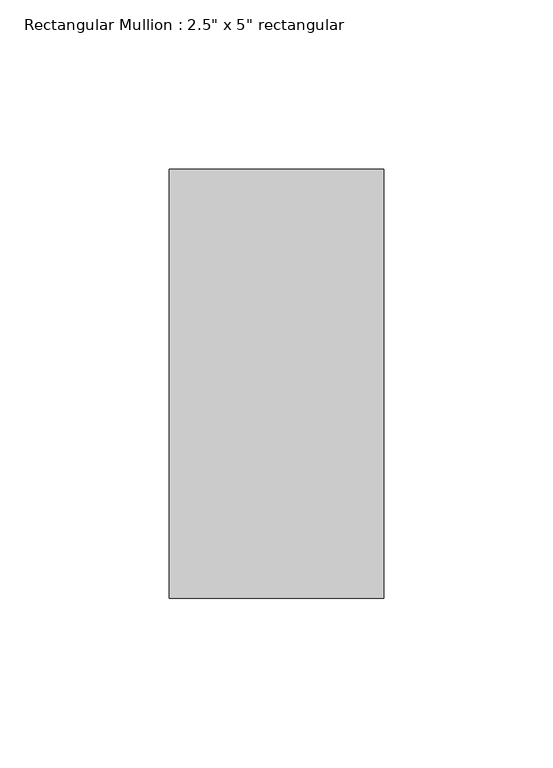
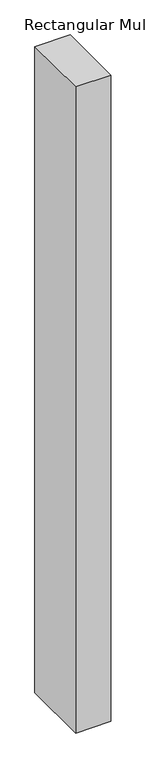
"""IFC4 building model written with IfcOpenShell, lengths in millimetres: member geometry."""

from ifc_helpers import new_model, si_unit, frame, origin, place, context, project, spatial, polyline, outline, extrude, source, transform, mapped, element, save


def member_b6df92ca(model_context):
    return source(origin(), model_context, "Body", "SweptSolid", [
        extrude(outline(polyline([(0.0, 63.5), (0.0, -63.5), (-63.5, -63.5), (-63.5, 63.5), (0.0, 63.5)])), frame((0.0, 0.0, -1231.8999998), z_axis=(0.0, 0.0, 1.0), x_axis=(1.0, 0.0, 0.0)), (0.0, 0.0, 1.0), 1231.8999998),
    ])


if __name__ == "__main__":
    model = new_model("IFC4")
    model_context = context("Model", 3, world=origin())
    ifc_project = project(units=[si_unit("LENGTHUNIT", "METRE", prefix="MILLI")], contexts=[model_context])
    site = spatial("IfcSite", under=ifc_project)
    building = spatial("IfcBuilding", under=site)
    placement = place(None, origin())
    member_shape = member_b6df92ca(model_context)
    element("IfcMember", 1, ObjectType="Rectangular Mullion : 2.5\" x 5\" rectangular", at=placement, inside=building, context=model_context, shape_type="MappedRepresentation", body=[
        mapped(member_shape, transform((0.0, 0.0, 0.0), x_axis=(1.0, 0.0, 0.0), y_axis=(0.0, 1.0, 0.0), z_axis=(0.0, 0.0, 1.0))),
    ])
    save(model, "model.ifc")

# Revit data of these elements
# Type "Rectangular Mullion : 2.5\" x 5\" rectangular"
#   built-in parameter 1007304 = 0.416667 (stored number, unit not read)
#   built-in parameter 1007301 = 0.104167 (stored number, unit not read)
#   built-in parameter 1007300 = 0.104167 (stored number, unit not read)
# Element 1 (IfcMember, "Rectangular Mullion : 2.5\" x 5\" rectangular")
#   Materials on its faces: "Aluminum"
# Materials
#   "Aluminum": class "Metal", colour RGB 247 247 247, transparency 0, Description = "Aluminum 6061", Cost = 0
